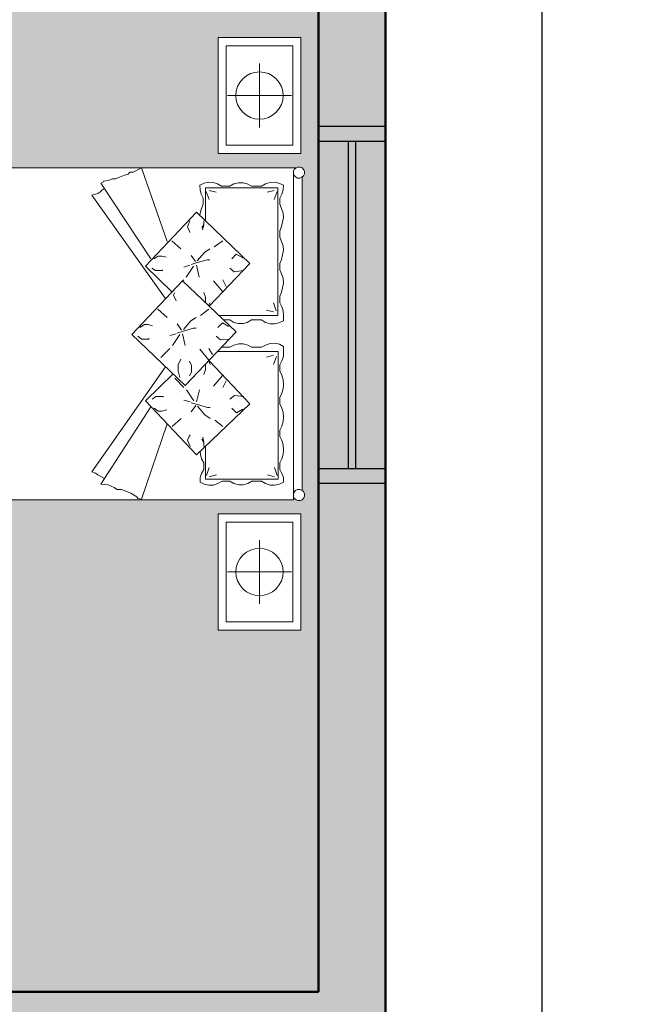
# Model space of a CAD drawing. Units: inches. Extents: x 528 to 2620, y -1066 to 798.
# Tile 33 of 41: x 1296 to 1381, y 524 to 656. Entities that reach past the tile are written whole.
import ezdxf

# ---------------------------------------------------------------- set-up
doc = ezdxf.new("R2010")
doc.units = ezdxf.units.IN
doc.header["$MEASUREMENT"] = 0
for name, color, linetype, lineweight in [('A-ANNO-DIMS', 2, 'Continuous', 18), ('A-FURN', 30, 'Continuous', 18), ('A-GLAZ', 3, 'Continuous', 25), ('A-WALL', 7, 'Continuous', 50), ('A-WALL-PATT', 8, 'Continuous', 13)]:
    doc.layers.add(name, color=color, linetype=linetype, lineweight=lineweight)
doc.styles.get("Standard").update_dxf_attribs({"font": 'arial.ttf'})
doc.dimstyles.get("Standard").update_dxf_attribs({"dimtxt": 6, "dimasz": 2, "dimexe": 0.18, "dimexo": 0.0625, "dimgap": 0.09, "dimtad": 0, "dimtih": 1, "dimtoh": 1, "dimdec": 1, "dimzin": 0, "dimdsep": 46, "dimlunit": 3, "dimtxsty": 'Standard', "dimblk": 'ARCHTICK', "dimcen": 0.09, "dimadec": 0, "dimazin": 0, "dimtfac": 1, "dimtdec": 1, "dimtofl": 0, "dimtmove": 0, "dimatfit": 3, "dimfxl": 1, "dimtolj": 1, "dimtzin": 0, "dimarcsym": 0})

# ---------------------------------------------------------------- blocks, each defined once
blk = doc.blocks.new('d-bed-3')
at = {"color": 0, "linetype": 'ByBlock'}
for p, q in [((0, 0), (0, -0.5)), ((0.7, 0), (0, 0)), ((0.7, -0.5), (0.7, 0)), ((0.7817, -0.0054), (0.7857, 0.0078)), ((0.7817, -0.0054), (0.7857, 0.0078)), ((0.7857, 0.0078), (0.7968, 0.0166)), ((0.7857, 0.0078), (0.7968, 0.0166)), ((0.7968, 0.0166), (0.8078, 0.0211)), ((0.7968, 0.0166), (0.8078, 0.0211)), ((0.8078, 0.0211), (0.8209, 0.0211)), ((0.8078, 0.0211), (0.8209, 0.0211)), ((0.8209, 0.0211), (0.8349, 0.0144)), ((0.8209, 0.0211), (0.8349, 0.0144)), ((0.8349, 0.0144), (0.8409, 0.0078)), ((0.8349, 0.0144), (0.8429, 0.0056)), ((0.8389, 0.0078), (2.7305, 0.0078)), ((0.8409, 0.0078), (2.7305, 0.0078)), ((0.8429, 0.0056), (0.848, -0.0077)), ((2.7234, -0.0077), (2.7284, 0.0056)), ((2.7284, 0.0056), (2.7365, 0.0144)), ((2.7305, 0.0078), (2.7365, 0.0144)), ((2.7365, 0.0144), (2.7505, 0.0211)), ((2.7365, 0.0144), (2.7505, 0.0211)), ((2.7505, 0.0211), (2.7636, 0.0211)), ((2.7505, 0.0211), (2.7636, 0.0211)), ((2.7636, 0.0211), (2.7746, 0.0166)), ((2.7636, 0.0211), (2.7746, 0.0166)), ((2.7746, 0.0166), (2.7857, 0.0078)), ((2.7746, 0.0166), (2.7857, 0.0078)), ((2.7857, 0.0078), (2.7897, -0.0054)), ((2.7857, 0.0078), (2.7897, -0.0054)), ((2.8714, -0.5), (2.8714, 0)), ((2.8714, 0), (3.5714, 0)), ((3.5714, 0), (3.5714, -0.5)), ((0.05, -0.05), (0.05, -0.45)), ((0.65, -0.05), (0.05, -0.05)), ((0.35, -0.0576), (0.35, -0.4424)), ((0.65, -0.45), (0.65, -0.05)), ((0.7817, -0.0187), (0.7817, -0.0054)), ((0.7817, -0.0187), (0.7817, -0.0054)), ((0.7857, -0.0297), (0.7817, -0.0187)), ((0.7857, -0.0297), (0.7817, -0.0187)), ((0.7857, -2.0939), (0.7857, -0.0297)), ((0.7948, -0.0408), (0.7857, -0.0297)), ((0.7857, -0.032), (0.7857, -2.0939)), ((0.8058, -0.0452), (0.7948, -0.0408)), ((0.8188, -0.0452), (0.8058, -0.0452)), ((0.8319, -0.0408), (0.8188, -0.0452)), ((2.7525, -0.0452), (0.8188, -0.0452)), ((0.8409, -0.032), (0.8319, -0.0408)), ((0.848, -0.0209), (0.8409, -0.032)), ((0.848, -0.0077), (0.848, -0.0209)), ((2.7234, -0.0209), (2.7234, -0.0077)), ((2.7305, -0.032), (2.7234, -0.0209)), ((2.7395, -0.0408), (2.7305, -0.032)), ((2.7525, -0.0452), (2.7395, -0.0408)), ((2.7656, -0.0452), (2.7525, -0.0452)), ((2.7766, -0.0408), (2.7656, -0.0452)), ((2.7766, -0.0408), (2.7656, -0.0452)), ((2.7656, -0.0452), (2.7857, -0.0452)), ((2.7857, -0.0452), (2.7656, -0.0452)), ((2.7857, -0.0297), (2.7766, -0.0408)), ((2.7857, -0.0297), (2.7766, -0.0408)), ((2.7897, -0.0187), (2.7857, -0.0297)), ((2.7897, -0.0187), (2.7857, -0.0297)), ((2.7857, -2.0939), (2.7857, -0.0452)), ((2.7897, -0.0054), (2.7897, -0.0187)), ((2.7897, -0.0054), (2.7897, -0.0187)), ((2.9214, -0.45), (2.9214, -0.05)), ((2.9214, -0.05), (3.5214, -0.05)), ((3.2214, -0.0576), (3.2214, -0.4424)), ((3.5214, -0.05), (3.5214, -0.45)), ((0.8781, -0.1325), (0.8911, -0.1059)), ((0.8911, -0.1059), (0.9182, -0.1082)), ((0.9182, -0.1082), (0.9443, -0.1148)), ((0.9443, -0.1148), (0.9684, -0.128)), ((1.0056, -0.128), (1.0317, -0.117)), ((1.0317, -0.117), (1.0588, -0.1082)), ((1.0588, -0.1082), (1.0849, -0.1059)), ((1.0849, -0.1059), (1.113, -0.1104)), ((1.113, -0.1104), (1.1401, -0.117)), ((1.1401, -0.117), (1.1662, -0.128)), ((1.2034, -0.128), (1.2295, -0.117)), ((1.2295, -0.117), (1.2566, -0.1082)), ((1.2566, -0.1082), (1.2827, -0.1059)), ((1.2827, -0.1059), (1.3108, -0.1104)), ((1.3108, -0.1104), (1.3379, -0.117)), ((1.3379, -0.117), (1.362, -0.128)), ((1.4012, -0.128), (1.4253, -0.117)), ((1.4253, -0.117), (1.4514, -0.1082)), ((1.4514, -0.1082), (1.4805, -0.1059)), ((1.4805, -0.1059), (1.5086, -0.1104)), ((1.5086, -0.1104), (1.5357, -0.117)), ((1.5357, -0.117), (1.5598, -0.128)), ((1.5989, -0.128), (1.623, -0.1148)), ((1.623, -0.1148), (1.6471, -0.1082)), ((1.6471, -0.1082), (1.6763, -0.1059)), ((1.6763, -0.1059), (1.7084, -0.1059)), ((1.7084, -0.1059), (1.7194, -0.1325)), ((1.8489, -0.1302), (1.863, -0.1059)), ((1.863, -0.1059), (1.8951, -0.1059)), ((1.8951, -0.1059), (1.9222, -0.1059)), ((1.9222, -0.1059), (1.9483, -0.1148)), ((1.9483, -0.1148), (1.9724, -0.128)), ((2.0096, -0.128), (2.0357, -0.1148)), ((2.0357, -0.1148), (2.0628, -0.1082)), ((2.0628, -0.1082), (2.0909, -0.1059)), ((2.0909, -0.1059), (2.117, -0.1082)), ((2.117, -0.1082), (2.1441, -0.1148)), ((2.1441, -0.1148), (2.1702, -0.128)), ((2.2074, -0.128), (2.2335, -0.1148)), ((2.2335, -0.1148), (2.2606, -0.1082)), ((2.2606, -0.1082), (2.2867, -0.1059)), ((2.2867, -0.1059), (2.3148, -0.1082)), ((2.3148, -0.1082), (2.3419, -0.1148)), ((2.3419, -0.1148), (2.366, -0.128)), ((2.4052, -0.128), (2.4293, -0.1148)), ((2.4293, -0.1148), (2.4554, -0.1082)), ((2.4554, -0.1082), (2.4845, -0.1059)), ((2.4845, -0.1059), (2.5126, -0.1082)), ((2.5126, -0.1082), (2.5397, -0.1148)), ((2.5397, -0.1148), (2.5638, -0.128)), ((2.6029, -0.128), (2.627, -0.1148)), ((2.627, -0.1148), (2.6511, -0.1059)), ((2.6511, -0.1059), (2.6803, -0.1059)), ((2.6803, -0.1059), (2.6913, -0.1302)), ((0.8721, -0.159), (0.8781, -0.1325)), ((0.8741, -0.1866), (0.8721, -0.159)), ((0.9072, -0.5753), (0.9072, -0.1391)), ((0.9072, -0.1391), (1.6763, -0.1391)), ((0.9223, -0.1612), (0.9333, -0.2042)), ((0.9293, -0.1435), (0.9775, -0.1612)), ((0.9684, -0.128), (1.0056, -0.128)), ((1.1662, -0.128), (1.2034, -0.128)), ((1.362, -0.128), (1.4012, -0.128)), ((1.5598, -0.128), (1.5989, -0.128)), ((1.6471, -0.1501), (1.5989, -0.1656)), ((1.6542, -0.1656), (1.6431, -0.2087)), ((1.6763, -0.1391), (1.6763, -0.4936)), ((1.7194, -0.1325), (1.7265, -0.159)), ((1.7265, -0.159), (1.7265, -0.1866)), ((1.8429, -0.159), (1.8489, -0.1302)), ((1.8449, -0.1866), (1.8429, -0.159)), ((2.6622, -0.1369), (1.8931, -0.1369)), ((1.8931, -0.1369), (1.8931, -0.5046)), ((1.9152, -0.1656), (1.9263, -0.2087)), ((1.9222, -0.1479), (1.9704, -0.1656)), ((1.9724, -0.128), (2.0096, -0.128)), ((2.1702, -0.128), (2.2074, -0.128)), ((2.366, -0.128), (2.4052, -0.128)), ((2.5638, -0.128), (2.6029, -0.128)), ((2.6401, -0.1435), (2.5919, -0.159)), ((2.6471, -0.159), (2.6361, -0.202)), ((2.6622, -0.5753), (2.6622, -0.1369)), ((2.6913, -0.1302), (2.6973, -0.159)), ((2.6973, -0.159), (2.6973, -0.1866)), ((0.8831, -0.2131), (0.8741, -0.1866)), ((0.8962, -0.2374), (0.8831, -0.2131)), ((1.7174, -0.2131), (1.7024, -0.2374)), ((1.7265, -0.1866), (1.7174, -0.2131)), ((1.854, -0.2131), (1.8449, -0.1866)), ((1.867, -0.2374), (1.854, -0.2131)), ((2.6883, -0.2131), (2.6732, -0.2374)), ((2.6973, -0.1866), (2.6883, -0.2131)), ((0.1576, -0.25), (0.5424, -0.25)), ((0.8962, -0.2992), (0.8962, -0.2374)), ((1.7024, -0.2374), (1.7024, -0.2992)), ((1.867, -0.297), (1.867, -0.2374)), ((2.6732, -0.2374), (2.6732, -0.297)), ((3.4138, -0.25), (3.029, -0.25)), ((0.8761, -0.3489), (0.8831, -0.3235)), ((0.8761, -0.3776), (0.8761, -0.3489)), ((0.8831, -0.3235), (0.8962, -0.2992)), ((1.0538, -0.6294), (1.362, -0.3081)), ((1.3289, -0.3511), (1.3068, -0.3909)), ((1.362, -0.3081), (1.619, -0.5532)), ((1.4052, -0.3467), (1.4122, -0.4019)), ((1.7024, -0.2992), (1.7174, -0.3235)), ((1.7174, -0.3235), (1.7244, -0.3489)), ((1.7244, -0.3489), (1.7244, -0.3776)), ((1.8469, -0.3489), (1.854, -0.3213)), ((1.8469, -0.3754), (1.8469, -0.3489)), ((1.854, -0.3213), (1.867, -0.297)), ((2.2074, -0.3081), (1.9483, -0.5532)), ((2.1632, -0.3445), (2.1572, -0.3997)), ((2.5146, -0.6294), (2.2074, -0.3081)), ((2.2405, -0.3511), (2.2626, -0.3887)), ((2.6732, -0.297), (2.6883, -0.3213)), ((2.6883, -0.3213), (2.6953, -0.3489)), ((2.6953, -0.3489), (2.6953, -0.3754)), ((0.8831, -0.4041), (0.8761, -0.3776)), ((0.8962, -0.4284), (0.8831, -0.4041)), ((1.3068, -0.3909), (1.3349, -0.4174)), ((1.4122, -0.4019), (1.3901, -0.4284)), ((1.4674, -0.7134), (1.7746, -0.3909)), ((1.7174, -0.4041), (1.7024, -0.4284)), ((1.7244, -0.3776), (1.7174, -0.4041)), ((1.7746, -0.3909), (2.0979, -0.6979)), ((1.854, -0.4041), (1.8469, -0.3754)), ((1.867, -0.4284), (1.854, -0.4041)), ((2.1572, -0.3997), (2.1793, -0.4284)), ((2.2626, -0.3887), (2.2335, -0.4174)), ((2.6883, -0.4041), (2.6732, -0.4284)), ((2.6953, -0.3754), (2.6883, -0.4041)), ((0.05, -0.45), (0.65, -0.45)), ((0.8962, -0.4781), (0.8962, -0.4284)), ((1.2255, -0.4715), (1.2626, -0.5223)), ((1.5006, -0.4505), (1.4604, -0.4715)), ((1.5327, -0.4715), (1.4674, -0.5267)), ((1.7024, -0.4284), (1.7024, -0.4649)), ((1.7415, -0.4351), (1.7194, -0.4737)), ((1.7194, -0.4737), (1.7485, -0.5002)), ((1.8188, -0.4306), (1.8228, -0.4848)), ((1.867, -0.4781), (1.867, -0.4284)), ((2.0357, -0.4715), (2.102, -0.5267)), ((2.0688, -0.4505), (2.109, -0.4715)), ((2.3439, -0.4715), (2.3068, -0.5201)), ((2.6732, -0.4284), (2.6732, -0.4759)), ((3.5214, -0.45), (2.9214, -0.45)), ((0, -0.5), (0.7, -0.5)), ((0.8721, -0.5576), (0.8741, -0.5289)), ((0.8741, -0.5289), (0.8831, -0.5024)), ((0.8831, -0.5024), (0.8962, -0.4781)), ((0.9223, -0.5532), (0.9333, -0.5113)), ((1.8228, -0.4848), (1.8008, -0.5113)), ((1.9112, -0.5333), (1.874, -0.5554)), ((2.6471, -0.5532), (2.6361, -0.5091)), ((2.6732, -0.4759), (2.6883, -0.5002)), ((2.6883, -0.5002), (2.6973, -0.5267)), ((2.6973, -0.5267), (2.6973, -0.5554)), ((3.5714, -0.5), (2.8714, -0.5)), ((0.8781, -0.5841), (0.8721, -0.5576)), ((0.8911, -0.6096), (0.8781, -0.5841)), ((1.109, -0.5753), (0.9072, -0.5753)), ((0.9293, -0.5709), (0.9775, -0.5532)), ((0.9684, -0.5886), (0.9443, -0.6007)), ((1.0056, -0.5886), (0.9684, -0.5886)), ((1.0317, -0.5996), (1.0056, -0.5886)), ((1.105, -0.5864), (1.1271, -0.5864)), ((1.1271, -0.5864), (1.1482, -0.5974)), ((1.1482, -0.5974), (1.1311, -0.5864)), ((1.1311, -0.5864), (1.1592, -0.593)), ((1.2957, -0.5819), (1.2737, -0.5488)), ((1.3459, -0.625), (1.2957, -0.5819)), ((1.3399, -0.5643), (1.3399, -0.5488)), ((1.357, -0.625), (1.3399, -0.5643)), ((1.5658, -0.5753), (1.5377, -0.5864)), ((1.5969, -0.5753), (1.5658, -0.5753)), ((1.5989, -0.5488), (1.614, -0.5554)), ((1.6381, -0.5554), (1.6763, -0.6051)), ((1.9443, -0.5554), (1.8781, -0.6096)), ((1.9704, -0.5466), (1.9503, -0.5554)), ((1.9684, -0.5753), (2.0036, -0.5753)), ((2.0036, -0.5753), (2.0317, -0.5864)), ((2.2124, -0.6228), (2.2295, -0.5643)), ((2.2224, -0.6228), (2.2736, -0.5797)), ((2.2295, -0.5643), (2.2295, -0.5466)), ((2.2736, -0.5797), (2.2957, -0.5466)), ((2.4383, -0.5864), (2.4092, -0.5908)), ((2.4423, -0.5864), (2.4202, -0.5974)), ((2.4202, -0.5974), (2.4383, -0.5864)), ((2.4644, -0.5864), (2.4423, -0.5864)), ((2.4604, -0.5753), (2.6622, -0.5753)), ((2.5638, -0.5864), (2.5397, -0.5996)), ((2.6029, -0.5864), (2.5638, -0.5864)), ((2.6401, -0.5687), (2.5919, -0.5532)), ((2.627, -0.5996), (2.6029, -0.5864)), ((2.6913, -0.5841), (2.6803, -0.6073)), ((2.6973, -0.5554), (2.6913, -0.5841)), ((0.9182, -0.6073), (0.8911, -0.6096)), ((0.9443, -0.6007), (0.9182, -0.6073)), ((1.0588, -0.6073), (1.0317, -0.5996)), ((1.3791, -0.9365), (1.0538, -0.6294)), ((1.0759, -0.6096), (1.0588, -0.6073)), ((1.3138, -0.6626), (1.351, -0.6361)), ((1.368, -0.6626), (1.357, -0.625)), ((1.3731, -0.6294), (1.4453, -0.614)), ((1.3791, -0.6471), (1.4453, -0.6913)), ((1.7084, -0.6648), (1.6873, -0.6316)), ((1.7526, -0.6493), (1.7526, -0.6316)), ((1.7706, -0.7089), (1.7526, -0.6493)), ((2.0387, -0.6427), (2.0427, -0.6405)), ((2.1963, -0.6294), (2.124, -0.6118)), ((2.1903, -0.6449), (2.124, -0.6891)), ((2.1903, -0.9365), (2.5146, -0.6294)), ((2.2013, -0.6626), (2.2124, -0.6228)), ((2.2556, -0.6626), (2.2184, -0.6338)), ((2.5126, -0.6051), (2.4955, -0.6073)), ((2.5397, -0.5996), (2.5126, -0.6051)), ((2.6511, -0.6073), (2.627, -0.5996)), ((2.6803, -0.6073), (2.6511, -0.6073)), ((1.105, -0.6692), (1.1421, -0.6846)), ((1.1421, -0.6846), (1.1642, -0.6736)), ((1.1642, -0.6736), (1.1753, -0.6692)), ((1.3731, -0.6692), (1.3841, -0.7067)), ((1.4674, -0.7134), (1.4604, -0.7067)), ((1.7596, -0.7089), (1.7084, -0.6648)), ((1.7817, -0.7454), (1.7706, -0.7089)), ((1.7857, -0.7134), (1.856, -0.6979)), ((2.0979, -0.6979), (1.7897, -1.0193)), ((1.9765, -0.6604), (1.9503, -0.6714)), ((2.0166, -0.6604), (1.9765, -0.6604)), ((2.0387, -0.6714), (2.0166, -0.6604)), ((2.0538, -0.7609), (2.109, -0.7067)), ((2.1963, -0.667), (2.1853, -0.7067)), ((2.4052, -0.6736), (2.3941, -0.667)), ((2.4272, -0.6846), (2.4052, -0.6736)), ((2.4644, -0.667), (2.4272, -0.6846)), ((1.2255, -0.7785), (1.2737, -0.7244)), ((1.7897, -1.0193), (1.4674, -0.7134)), ((1.5548, -0.7675), (1.5397, -0.7631)), ((1.5548, -0.7675), (1.5769, -0.7564)), ((1.5769, -0.7564), (1.5879, -0.752)), ((1.7265, -0.7454), (1.7636, -0.72)), ((1.7857, -0.752), (1.7967, -0.7896)), ((1.7897, -0.731), (1.856, -0.7741)), ((1.9724, -0.741), (1.9393, -0.7244)), ((2.0096, -0.741), (1.9724, -0.741)), ((2.0497, -0.731), (2.0096, -0.741)), ((2.1903, -0.9365), (2.0277, -0.7697)), ((2.3439, -0.7763), (2.2957, -0.7222)), ((0.7857, -0.9607), (1.2295, -0.8072)), ((0.9504, -1.2611), (1.5708, -0.8183)), ((1.3178, -0.8382), (1.3239, -0.8117)), ((1.3791, -0.9365), (1.5357, -0.7763)), ((1.6381, -0.8625), (1.6873, -0.8072)), ((1.9283, -0.8448), (1.874, -0.7896)), ((2.618, -1.2611), (1.9855, -0.8161)), ((2.2515, -0.8382), (2.2445, -0.8094)), ((2.7827, -0.9607), (2.3278, -0.8072)), ((1.3178, -0.8602), (1.3178, -0.8382)), ((1.3349, -0.8879), (1.3178, -0.8602)), ((1.3901, -0.8989), (1.4052, -0.8768)), ((1.4052, -0.8337), (1.4012, -0.8337)), ((1.4052, -0.8768), (1.4052, -0.8337)), ((2.1632, -0.8757), (2.1632, -0.8315)), ((2.1632, -0.8315), (2.1682, -0.8315)), ((2.1793, -0.8967), (2.1632, -0.8757)), ((2.2335, -0.8856), (2.2515, -0.8602)), ((2.2515, -0.8602), (2.2515, -0.8382)), ((0.8781, -1.2059), (1.3349, -0.9055)), ((1.7305, -0.921), (1.7375, -0.8945)), ((1.7305, -0.9431), (1.7305, -0.921)), ((1.7485, -0.9718), (1.7305, -0.9431)), ((1.8188, -0.9166), (1.8118, -0.9166)), ((1.8188, -0.9607), (1.8188, -0.9166)), ((2.6913, -1.2059), (2.2254, -0.9055)), ((0.8128, -1.0115), (0.7857, -0.9607)), ((1.8008, -0.9828), (1.8188, -0.9607)), ((2.7676, -0.9895), (2.7455, -1.0259)), ((2.7786, -0.9828), (2.7676, -0.9895)), ((2.7827, -0.9607), (2.7786, -0.9828)), ((0.8128, -1.0325), (0.8128, -1.0115)), ((0.8239, -1.0414), (0.8128, -1.0325)), ((0.8299, -1.0635), (0.8239, -1.0414)), ((0.8349, -1.0745), (0.8299, -1.0635)), ((2.7455, -1.0259), (2.7234, -1.0811)), ((0.845, -1.1032), (0.8349, -1.0745)), ((0.852, -1.1187), (0.845, -1.1032)), ((0.852, -1.1363), (0.852, -1.1187)), ((2.7124, -1.1253), (2.6953, -1.1617)), ((2.7174, -1.1187), (2.7124, -1.1253)), ((2.7234, -1.1076), (2.7174, -1.1187)), ((2.7234, -1.0811), (2.7234, -1.1076)), ((0.863, -1.1617), (0.852, -1.1363)), ((0.867, -1.1905), (0.863, -1.1617)), ((0.9223, -1.2015), (0.9112, -1.1838)), ((2.6582, -1.1838), (2.6471, -1.2015)), ((2.6953, -1.1617), (2.6913, -1.2059)), ((0.8741, -1.1949), (0.867, -1.1905)), ((0.8781, -1.2059), (0.8741, -1.1949)), ((0.9293, -1.2059), (0.9223, -1.2015)), ((0.9403, -1.2236), (0.9293, -1.2059)), ((0.9443, -1.2391), (0.9403, -1.2236)), ((0.9504, -1.2611), (0.9443, -1.2391)), ((2.625, -1.2391), (2.618, -1.2611)), ((2.6361, -1.2236), (2.625, -1.2391)), ((2.6471, -1.2015), (2.6361, -1.2236)), ((2.7234, -2.0497), (2.6913, -1.947)), ((0.8741, -2.0673), (0.9464, -1.9691)), ((0.8851, -2.1005), (0.9795, -2.0342)), ((2.7305, -2.0939), (2.6421, -2.0342)), ((0.7797, -2.148), (0.7857, -2.1347)), ((0.7797, -2.148), (0.7857, -2.1347)), ((0.7888, -2.1317), (0.7857, -2.0939)), ((0.7857, -2.0939), (0.7887, -2.1303)), ((0.7857, -2.1347), (0.7948, -2.1259)), ((0.7857, -2.1347), (0.7888, -2.1317)), ((0.7948, -2.1259), (0.8078, -2.1215)), ((0.8078, -2.1215), (0.8188, -2.1215)), ((0.8188, -2.1215), (0.8319, -2.1281)), ((0.8319, -2.1281), (0.8409, -2.1369)), ((2.7365, -2.1281), (2.7284, -2.1369)), ((2.7505, -2.1215), (2.7365, -2.1281)), ((2.7616, -2.1215), (2.7505, -2.1215)), ((2.7746, -2.1259), (2.7616, -2.1215)), ((2.7827, -2.1347), (2.7746, -2.1259)), ((2.7857, -2.0939), (2.7783, -2.1299)), ((2.7783, -2.1299), (2.7827, -2.1347)), ((2.7786, -2.1281), (2.7857, -2.0939)), ((2.7827, -2.1347), (2.7897, -2.148)), ((2.7897, -2.148), (2.7827, -2.1347)), ((0.7797, -2.159), (0.7797, -2.148)), ((0.7797, -2.148), (0.7797, -2.159)), ((0.7837, -2.1723), (0.7797, -2.159)), ((0.7837, -2.1723), (0.7797, -2.159)), ((0.7927, -2.1811), (0.7837, -2.1723)), ((0.7927, -2.1811), (0.7837, -2.1723)), ((0.8058, -2.1877), (0.7927, -2.1811)), ((0.8058, -2.1877), (0.7927, -2.1811)), ((0.8168, -2.1877), (0.8058, -2.1877)), ((0.8168, -2.1877), (0.8058, -2.1877)), ((0.8299, -2.1833), (0.8168, -2.1877)), ((0.8299, -2.1833), (0.8168, -2.1877)), ((0.8389, -2.1745), (0.8299, -2.1833)), ((0.8367, -2.1767), (0.8299, -2.1833)), ((2.7327, -2.1767), (0.8367, -2.1767)), ((0.845, -2.1612), (0.8389, -2.1745)), ((0.8389, -2.1767), (2.7305, -2.1767)), ((0.8409, -2.1369), (0.845, -2.1502)), ((2.7264, -2.1436), (0.845, -2.1436)), ((0.845, -2.1502), (0.845, -2.1612)), ((2.7284, -2.1369), (2.7234, -2.1502)), ((2.7234, -2.1502), (2.7234, -2.1612)), ((2.7234, -2.1612), (2.7305, -2.1745)), ((2.7305, -2.1745), (2.7395, -2.1833)), ((2.7395, -2.1833), (2.7327, -2.1767)), ((2.7525, -2.1877), (2.7395, -2.1833)), ((2.7395, -2.1833), (2.7525, -2.1877)), ((2.7636, -2.1877), (2.7525, -2.1877)), ((2.7525, -2.1877), (2.7636, -2.1877)), ((2.7766, -2.1811), (2.7636, -2.1877)), ((2.7636, -2.1877), (2.7766, -2.1811)), ((2.7857, -2.1723), (2.7766, -2.1811)), ((2.7766, -2.1811), (2.7857, -2.1723)), ((2.7897, -2.159), (2.7857, -2.1723)), ((2.7857, -2.1723), (2.7897, -2.159)), ((2.7897, -2.148), (2.7897, -2.159)), ((2.7897, -2.159), (2.7897, -2.148))]:
    blk.add_line(p, q, dxfattribs=at)
blk.add_ellipse((0.35, -0.25), major_axis=(-0.1007, 0.1007), ratio=1, dxfattribs=at)
at = {"color": 0, "linetype": 'ByBlock', "extrusion": (0, 0, -1)}
blk.add_ellipse((3.2214, -0.25), major_axis=(0.1007, 0.1007), ratio=1, dxfattribs=at)
blk = doc.blocks.new('_ArchTick')
at = {"color": 0, "linetype": 'ByBlock', "const_width": 0.15}
blk.add_lwpolyline([(-0.5, -0.5), (0.5, 0.5)], dxfattribs=at)
blk = doc.blocks.new('*D17')
at = {"layer": 'A-ANNO-DIMS', "color": 0, "lineweight": -2, "transparency": 16777216}
for p, q in [((1345.06, 718.92), (1366.18, 718.92)), ((1366, 718.92), (1366, 497.08)), ((1366, 268.92), (1366, 490.77)), ((1345.06, 268.92), (1366.18, 268.92))]:
    blk.add_line(p, q, dxfattribs=at)
at = {"layer": 'Defpoints', "color": 0, "transparency": 16777216}
for p in [(1345, 718.92), (1345, 268.92), (1366, 268.92)]:
    blk.add_point(p, dxfattribs=at)
at = {"layer": 'A-ANNO-DIMS', "color": 0, "lineweight": -2, "transparency": 16777216, "xscale": 2, "yscale": 2, "zscale": 2}
for p, rotation in [((1366, 718.92), 90), ((1366, 268.92), 270)]:
    blk.add_blockref('_ArchTick', p, dxfattribs=dict(at, rotation=rotation))
at = {"layer": 'A-ANNO-DIMS', "color": 0, "transparency": 16777216, "insert": (1366, 493.92), "char_height": 6, "attachment_point": 5}
blk.add_mtext('\\A1;37\'-6.0"', dxfattribs=at)
blk = doc.blocks.new('WIN-1200')
for p, q in [((677.56, 718.92), (725.56, 718.92)), ((677.56, 709.92), (677.56, 718.92)), ((679.56, 709.92), (679.56, 718.92)), ((723.56, 718.92), (723.56, 709.92)), ((725.56, 718.92), (725.56, 709.92)), ((679.56, 714.92), (723.56, 714.92)), ((679.56, 713.92), (723.56, 713.92)), ((725.56, 709.92), (677.56, 709.92))]:
    blk.add_line(p, q)

msp = doc.modelspace()

# ---------------------------------------------------------------- hatches: boundary and pattern name
at = {"layer": 'A-WALL-PATT', "transparency": 33554521}
h = msp.add_hatch(color=256, dxfattribs=at)
h.dxf.hatch_style = 1
h.paths.add_polyline_path([(1066, 709.92), (1114.5, 709.92), (1114.5, 718.92), (1057, 718.92), (1057, 667.92), (1066, 667.92)])
h.paths.add_polyline_path([(1227.5, 718.92), (1162.5, 718.92), (1162.5, 709.92), (1211, 709.92), (1211, 577.92), (1205.42, 577.92), (1205.5, 573.42), (1211, 573.42), (1211, 567.42), (1215.5, 567.42), (1215.5, 669.42), (1268, 669.42), (1268, 675.92), (1263.5, 675.92), (1263.5, 673.92), (1215.5, 673.92), (1215.5, 709.92), (1227.5, 709.92)])
h.paths.add_polyline_path([(1345, 718.92), (1316, 718.92), (1316, 709.92), (1336, 709.92), (1336, 641.67), (1345, 641.67)])
h.paths.add_polyline_path([(1066, 619.92), (1057, 619.92), (1057, 561.42), (1066, 561.42), (1066, 573.42), (1161, 573.42), (1161, 569.42), (1165.5, 569.42), (1165.5, 577.92), (1066, 577.92)])
h.paths.add_polyline_path([(1216, 391.42), (1216, 400.42), (1207, 400.42), (1201, 400.42), (1201, 397.42), (1201, 391.42), (1207, 391.42), (1207, 268.92), (1252, 268.92), (1252, 277.92), (1216, 277.92), (1216, 359.77)])
h.paths.add_polyline_path([(1345, 395.92), (1336, 395.92), (1288, 395.92), (1288, 391.42), (1336, 391.42), (1336, 277.92), (1300, 277.92), (1300, 268.92), (1345, 268.92)])
h.paths.add_polyline_path([(1345, 593.67), (1336, 593.67), (1336, 525.42), (1215.5, 525.42), (1215.5, 527.17), (1211, 527.17), (1211, 520.92), (1336, 520.92), (1336, 443.92), (1345, 443.92)])
h.paths.add_polyline_path([(1066, 520.92), (1165.5, 520.92), (1165.5, 545.42), (1161, 545.42), (1161, 525.42), (1066, 525.42), (1066, 537.42), (1057, 537.42), (1057, 484.67), (1066, 484.67)])
h.paths.add_polyline_path([(1066, 436.67), (1057, 436.67), (1057, 391.42), (1085.5, 391.42), (1085.5, 400.42), (1066, 400.42)])
h.paths.add_polyline_path([(1153, 397.42), (1153, 400.42), (1133.5, 400.42), (1133.5, 391.42), (1153, 391.42)])
at = {"layer": 'A-WALL-PATT', "transparency": 33554681}
h = msp.add_hatch(color=256, dxfattribs=at)
h.dxf.hatch_style = 1
h.paths.add_polyline_path([(1066, 665.92), (1062, 665.92), (1062, 621.92), (1066, 621.92)])
h.paths.add_polyline_path([(1061, 665.92), (1057, 665.92), (1057, 621.92), (1061, 621.92)])
h.paths.add_polyline_path([(1160.5, 713.92), (1116.5, 713.92), (1116.5, 709.92), (1160.5, 709.92)])
h.paths.add_polyline_path([(1160.5, 718.92), (1116.5, 718.92), (1116.5, 714.92), (1160.5, 714.92)])
h.paths.add_polyline_path([(1251.5, 713.92), (1227.5, 713.92), (1227.5, 709.92), (1251.5, 709.92)])
h.paths.add_polyline_path([(1251.5, 718.92), (1227.5, 718.92), (1227.5, 714.92), (1251.5, 714.92)])
h.paths.add_polyline_path([(1314, 713.92), (1270, 713.92), (1270, 709.92), (1314, 709.92)])
h.paths.add_polyline_path([(1314, 718.92), (1270, 718.92), (1270, 714.92), (1314, 714.92)])
h.paths.add_polyline_path([(1345, 639.67), (1341, 639.67), (1341, 595.67), (1345, 595.67)])
h.paths.add_polyline_path([(1340, 639.67), (1336, 639.67), (1336, 595.67), (1340, 595.67)])
h.paths.add_polyline_path([(1345, 441.92), (1341, 441.92), (1341, 397.92), (1345, 397.92)])
h.paths.add_polyline_path([(1340, 441.92), (1336, 441.92), (1336, 397.92), (1340, 397.92)])
h.paths.add_polyline_path([(1298, 272.92), (1254, 272.92), (1254, 268.92), (1298, 268.92)])
h.paths.add_polyline_path([(1298, 277.92), (1254, 277.92), (1254, 273.92), (1298, 273.92)])
h.paths.add_polyline_path([(1131.5, 395.42), (1087.5, 395.42), (1087.5, 391.42), (1131.5, 391.42)])
h.paths.add_polyline_path([(1131.5, 400.42), (1087.5, 400.42), (1087.5, 396.42), (1131.5, 396.42)])
h.paths.add_polyline_path([(1066, 482.67), (1062, 482.67), (1062, 438.67), (1066, 438.67)])
h.paths.add_polyline_path([(1061, 482.67), (1057, 482.67), (1057, 438.67), (1061, 438.67)])
h.paths.add_polyline_path([(1066, 561.42), (1062, 561.42), (1062, 537.42), (1066, 537.42)])
h.paths.add_polyline_path([(1061, 561.42), (1057, 561.42), (1057, 537.42), (1061, 537.42)])
at = {"layer": 'A-WALL-PATT', "transparency": 33554536}
h = msp.add_hatch(color=256, dxfattribs=at)
h.dxf.hatch_style = 1
h.paths.add_polyline_path([(1336, 709.92), (1268, 709.92), (1268, 699.92), (1266.75, 699.92), (1266.75, 675.92), (1268, 675.92), (1268, 669.42), (1215.5, 669.42), (1215.5, 567.17), (1217, 567.17), (1257, 567.17), (1257, 565.42), (1256.96, 565.42, -0.401453), (1217, 527.17), (1215.5, 527.17), (1215.5, 525.42), (1336, 525.42)], flags=17)
h.paths.add_polyline_path([(1285.03, 635.93), (1285.23, 636.13), (1285.67, 636.26), (1286.21, 636.02), (1286.98, 636.08), (1332.98, 636.08), (1333.36, 636.22), (1333.82, 636.08), (1334.11, 635.71), (1334.11, 635.3), (1333.91, 634.86), (1333.82, 634.83), (1333.82, 592.74), (1333.97, 592.6), (1334.11, 592.29), (1334.11, 591.88), (1333.82, 591.51), (1333.36, 591.37), (1332.98, 591.51), (1332.64, 591.79), (1332.64, 591.51), (1286.98, 591.51), (1286.17, 591.67), (1286.07, 591.57), (1285.68, 591.37), (1285.23, 591.51), (1285.03, 591.71), (1284.83, 592.1), (1284.98, 592.54), (1285.13, 592.69), (1285.13, 634.95), (1284.98, 635.1), (1284.83, 635.54)], flags=16)
h.paths.add_polyline_path([(1285.03, 635.93), (1285.23, 636.13), (1285.67, 636.26), (1286.21, 636.02), (1286.98, 636.08), (1332.98, 636.08), (1333.36, 636.22), (1333.82, 636.08), (1334.11, 635.71), (1334.11, 635.3), (1333.97, 634.99), (1333.82, 634.85), (1333.82, 592.74), (1333.97, 592.6), (1334.11, 592.29), (1334.11, 591.88), (1333.82, 591.51), (1333.36, 591.37), (1332.98, 591.51), (1332.64, 591.79), (1332.64, 592.25), (1332.64, 635.35), (1332.64, 635.8), (1332.98, 636.08), (1312.23, 636.08), (1311.1, 635.48), (1310.63, 635.48), (1310.43, 635.23), (1309.94, 635.1), (1309.7, 634.99), (1309.06, 634.76), (1308.71, 634.61), (1308.32, 634.61), (1307.75, 634.36), (1307.11, 634.27), (1307.01, 634.11), (1306.77, 634.02), (1307.25, 633.28), (1306.87, 633.04), (1306.77, 632.88), (1306.37, 632.64), (1306.03, 632.55), (1305.54, 632.41), (1315.47, 618.49), (1316.32, 619.39), (1312.77, 622.86), (1319.62, 630.11), (1320.07, 629.68), (1320.11, 630), (1320.28, 630.6), (1320.53, 631.18), (1320.53, 632.01), (1320.26, 632.55), (1320.11, 633.13), (1320.06, 633.73), (1320.63, 634.02), (1321.22, 634.16), (1321.86, 634.11), (1322.45, 633.91), (1322.99, 633.62), (1324.1, 633.62), (1324.64, 633.91), (1325.23, 634.07), (1325.87, 634.07), (1326.43, 633.91), (1326.98, 633.62), (1328.35, 633.62), (1328.9, 633.91), (1329.49, 634.11), (1330.1, 634.16), (1330.69, 634.02), (1331.28, 633.73), (1331.23, 633.13), (1331.09, 632.55), (1330.79, 632.01), (1330.79, 631.18), (1331.04, 630.6), (1331.23, 630), (1331.28, 629.41), (1331.19, 628.79), (1331.04, 628.18), (1330.79, 627.6), (1330.79, 626.77), (1331.04, 626.19), (1331.23, 625.59), (1331.28, 625.01), (1331.19, 624.38), (1331.04, 623.78), (1330.79, 623.24), (1330.79, 622.37), (1331.04, 621.83), (1331.23, 621.25), (1331.28, 620.6), (1331.19, 619.97), (1331.04, 619.37), (1330.79, 618.83), (1330.79, 617.96), (1331.09, 617.42), (1331.23, 616.88), (1331.28, 616.23), (1331.28, 615.52), (1330.69, 615.27), (1330.1, 615.12), (1329.49, 615.12), (1328.9, 615.32), (1328.35, 615.65), (1326.98, 615.65), (1326.43, 615.32), (1325.87, 615.16), (1325.23, 615.16), (1324.64, 615.32), (1324.1, 615.65), (1323.24, 615.65), (1324.93, 614.04), (1322.98, 611.98), (1324.1, 611.98), (1324.64, 612.27), (1325.28, 612.43), (1325.87, 612.43), (1326.48, 612.27), (1327.03, 611.98), (1328.35, 611.98), (1328.9, 612.27), (1329.49, 612.48), (1330.1, 612.52), (1330.74, 612.39), (1331.28, 612.07), (1331.28, 611.36), (1331.28, 610.75), (1331.09, 610.17), (1330.79, 609.63), (1330.79, 608.81), (1331.09, 608.22), (1331.23, 607.62), (1331.28, 606.99), (1331.23, 606.41), (1331.09, 605.81), (1330.79, 605.22), (1330.79, 604.4), (1331.09, 603.81), (1331.23, 603.21), (1331.28, 602.63), (1331.23, 602), (1331.09, 601.4), (1330.79, 600.86), (1330.79, 599.99), (1331.09, 599.45), (1331.23, 598.87), (1331.28, 598.22), (1331.23, 597.59), (1331.09, 596.99), (1330.79, 596.45), (1330.79, 595.58), (1331.09, 595.04), (1331.28, 594.51), (1331.28, 593.86), (1330.74, 593.61), (1330.1, 593.48), (1329.49, 593.48), (1328.9, 593.68), (1328.35, 594.01), (1327.03, 594.01), (1326.48, 593.68), (1325.87, 593.52), (1325.28, 593.52), (1324.64, 593.68), (1324.1, 594.01), (1323.04, 594.01), (1322.5, 593.68), (1321.91, 593.48), (1321.27, 593.48), (1320.63, 593.61), (1320.11, 593.86), (1320.11, 594.51), (1320.28, 595.04), (1320.58, 595.58), (1320.58, 596.45), (1320.28, 596.99), (1320.16, 597.59), (1320.1, 598.01), (1319.62, 597.55), (1315.66, 601.73), (1312.23, 591.57), (1311.74, 591.66), (1311.59, 591.91), (1310.78, 592.4), (1309.55, 592.89), (1308.96, 592.89), (1308.71, 593.03), (1308.56, 593.14), (1307.75, 593.52), (1306.77, 593.61), (1307.25, 594.36), (1306.87, 594.6), (1306.37, 594.84), (1306.03, 595.09), (1305.54, 595.24), (1315.46, 609.35), (1310.93, 613.71), (1315.47, 618.49), (1305.54, 632.41), (1306.03, 632.55), (1306.37, 632.64), (1306.77, 632.88), (1306.87, 633.04), (1307.25, 633.28), (1306.77, 634.02), (1307.01, 634.11), (1307.11, 634.27), (1307.75, 634.36), (1308.32, 634.61), (1308.71, 634.61), (1309.06, 634.76), (1309.7, 634.99), (1309.94, 635.1), (1310.43, 635.23), (1310.63, 635.48), (1311.1, 635.48), (1312.23, 636.08), (1286.98, 636.08), (1286.22, 636.02), (1286.41, 635.44), (1286.21, 635.05), (1286.02, 634.85), (1285.87, 634.81), (1285.87, 592.84), (1286.15, 592.73), (1286.41, 592.19), (1286.23, 591.66), (1286.17, 591.67), (1286.07, 591.57), (1285.68, 591.37), (1285.23, 591.51), (1285.03, 591.71), (1284.83, 592.1), (1284.98, 592.54), (1285.13, 592.69), (1285.13, 634.95), (1284.98, 635.1), (1284.83, 635.54)], flags=0)
h.paths.add_polyline_path([(1322.5, 653.6), (1333.65, 653.6), (1333.65, 637.99), (1322.5, 637.99)], flags=16)
h.paths.add_polyline_path([(1323.62, 652.48), (1332.53, 652.48), (1332.53, 639.11), (1323.62, 639.11)], flags=0)
edge = h.paths.add_edge_path(flags=0)
edge.add_ellipse((1328.07, 645.79), major_axis=(2.24, 2.24), ratio=1, start_angle=405, end_angle=495, ccw=False)
edge.add_ellipse((1328.07, 645.79), major_axis=(2.24, 2.24), ratio=1, start_angle=675, end_angle=765, ccw=False)
edge.add_ellipse((1328.07, 645.79), major_axis=(2.24, 2.24), ratio=1, start_angle=585, end_angle=675, ccw=False)
edge.add_ellipse((1328.07, 645.79), major_axis=(2.24, 2.24), ratio=1, start_angle=495, end_angle=585, ccw=False)
h.paths.add_polyline_path([(1320.58, 628.39), (1320.33, 628.01), (1320.61, 628.55)], flags=0)
h.paths.add_polyline_path([(1317.89, 604.89), (1318.78, 604.64), (1319.76, 604.28), (1318.88, 604.53)], flags=0)
h.paths.add_polyline_path([(1320.33, 599.65), (1320.58, 599.25), (1320.58, 599.16)], flags=0)
h.paths.add_polyline_path([(1322.5, 589.6), (1333.65, 589.6), (1333.65, 573.99), (1322.5, 573.99)], flags=16)
h.paths.add_polyline_path([(1323.62, 588.48), (1332.53, 588.48), (1332.53, 575.11), (1323.62, 575.11)], flags=0)
edge = h.paths.add_edge_path(flags=0)
edge.add_ellipse((1328.07, 581.8), major_axis=(-2.24, 2.24), ratio=1, start_angle=-45, end_angle=45, ccw=False)
edge.add_ellipse((1328.07, 581.8), major_axis=(-2.24, 2.24), ratio=1, start_angle=-135, end_angle=-45, ccw=False)
edge.add_ellipse((1328.07, 581.8), major_axis=(-2.24, 2.24), ratio=1, start_angle=135, end_angle=-135, ccw=False)
edge.add_ellipse((1328.07, 581.8), major_axis=(-2.24, 2.24), ratio=1, start_angle=45, end_angle=135, ccw=False)
h.paths.add_polyline_path([(1264.75, 699.92), (1263.5, 699.92), (1263.5, 709.92), (1215.5, 709.92), (1215.5, 673.92), (1263.5, 673.92), (1263.5, 675.92), (1264.75, 675.92)], flags=16)
h.paths.add_polyline_path([(1162.19, 569.42), (1161, 569.42), (1161, 573.42), (1066, 573.42), (1066, 525.42), (1161, 525.42), (1161, 545.42), (1162.19, 545.42)])
h.paths.add_polyline_path([(1256.96, 565.42), (1257, 565.42), (1257, 567.17), (1217, 567.17), (1215.5, 567.17), (1215.5, 567.42), (1211, 567.42), (1211, 573.42), (1205.5, 573.42), (1205.42, 577.92), (1211, 577.92), (1211, 709.92), (1066, 709.92), (1066, 577.92), (1165.5, 577.92), (1165.5, 569.42), (1164.19, 569.42), (1164.19, 545.42), (1165.5, 545.42), (1165.5, 520.92), (1153, 520.92), (1153, 484.92), (1102, 484.92), (1102, 436.42), (1153, 436.42), (1153, 400.42), (1153, 391.42), (1201, 391.42), (1201, 400.42), (1207, 400.42), (1216, 400.42), (1216, 391.42), (1216, 277.92), (1336, 277.92), (1336, 391.42), (1288, 391.42), (1288, 395.92), (1336, 395.92), (1336, 443.92), (1336, 520.92), (1211, 520.92), (1211, 527.17), (1215.5, 527.17), (1217, 527.17, 0.401453)])
h.paths.add_polyline_path([(1167.25, 579.42), (1165.5, 579.42), (1165.5, 619.42), (1167.25, 619.42)], flags=16)
h.paths.add_polyline_path([(1227.97, 501.56), (1236.36, 502.03), (1236.36, 492.55), (1227.97, 493.02, -0.254069)], flags=16)
h.paths.add_polyline_path([(1243.34, 515.69, -0.254069), (1251.88, 515.69), (1252.35, 507.3), (1242.87, 507.3)], flags=16)
h.paths.add_polyline_path([(1239.18, 504.68), (1256.03, 504.68), (1256.03, 479.42), (1239.18, 479.42)], flags=16)
h.paths.add_polyline_path([(1227.97, 489.6), (1236.36, 490.07), (1236.36, 480.59), (1227.97, 481.06, -0.254069)], flags=16)
h.paths.add_polyline_path([(1197.2, 624.04), (1197.2, 639.64), (1208.35, 639.64), (1208.35, 624.04)], flags=16)
h.paths.add_polyline_path([(1198.32, 625.15), (1198.32, 638.53), (1207.23, 638.53), (1207.23, 625.15)], flags=0)
h.paths.add_polyline_path([(1258.85, 502.03), (1267.25, 501.56, -0.254069), (1267.25, 493.02), (1258.85, 492.55)], flags=16)
h.paths.add_polyline_path([(1271.59, 519.66), (1333.67, 519.66), (1333.67, 451.59), (1319.09, 451.59), (1319.09, 505.07), (1288.09, 505.07), (1284.45, 505.07, -0.883215), (1270.68, 514.19), (1270.68, 518.75, -0.414214)], flags=16)
h.paths.add_polyline_path([(1331.85, 517.83), (1331.85, 453.42), (1328.2, 453.42), (1328.2, 505.07), (1298.42, 505.07), (1298.42, 514.19), (1288.09, 514.19), (1288.09, 517.83)], flags=0)
h.paths.add_polyline_path([(1242.87, 476.8), (1252.35, 476.8), (1251.88, 468.41, -0.254069), (1243.34, 468.41)], flags=16)
h.paths.add_polyline_path([(1258.85, 490.07), (1267.25, 489.6, -0.254069), (1267.25, 481.06), (1258.85, 480.59)], flags=16)
h.paths.add_polyline_path([(1161.68, 641.55), (1160.87, 641.72), (1160.77, 641.62), (1160.38, 641.41), (1159.93, 641.55), (1159.73, 641.75), (1159.53, 642.14), (1159.68, 642.58), (1159.83, 642.73), (1159.83, 684.99), (1159.68, 685.14), (1159.53, 685.58), (1159.73, 685.97), (1159.93, 686.17), (1160.37, 686.31), (1160.91, 686.06), (1161.68, 686.13), (1207.68, 686.13), (1208.06, 686.27), (1208.52, 686.13), (1208.81, 685.76), (1208.81, 685.34), (1208.61, 684.9), (1208.52, 684.87), (1208.52, 642.78), (1208.67, 642.65), (1208.88, 642.2), (1208.72, 641.8), (1208.52, 641.55), (1208.06, 641.41), (1207.68, 641.55), (1207.34, 641.83), (1207.34, 641.55)], flags=16)
h.paths.add_polyline_path([(1186.93, 641.62), (1186.44, 641.71), (1186.29, 641.95), (1185.48, 642.45), (1184.25, 642.94), (1183.66, 642.94), (1183.41, 643.07), (1183.26, 643.18), (1182.45, 643.57), (1181.47, 643.65), (1181.95, 644.4), (1181.57, 644.64), (1181.07, 644.89), (1180.73, 645.13), (1180.24, 645.29), (1190.16, 659.4), (1185.63, 663.75), (1190.17, 668.54), (1180.24, 682.46), (1180.73, 682.59), (1181.07, 682.68), (1181.47, 682.93), (1181.57, 683.08), (1181.95, 683.33), (1181.47, 684.07), (1181.71, 684.16), (1181.81, 684.31), (1182.45, 684.4), (1183.02, 684.65), (1183.41, 684.65), (1183.76, 684.81), (1184.4, 685.03), (1184.64, 685.14), (1185.13, 685.28), (1185.33, 685.52), (1185.8, 685.52), (1186.93, 686.13), (1161.68, 686.13), (1160.92, 686.06), (1161.11, 685.49), (1160.91, 685.1), (1160.72, 684.9), (1160.57, 684.85), (1160.57, 642.88), (1160.85, 642.77), (1161.11, 642.23), (1160.93, 641.7), (1160.87, 641.72), (1160.77, 641.62), (1160.38, 641.41), (1159.93, 641.55), (1159.73, 641.75), (1159.53, 642.14), (1159.68, 642.58), (1159.83, 642.73), (1159.83, 684.99), (1159.68, 685.14), (1159.53, 685.58), (1159.73, 685.97), (1159.93, 686.17), (1160.37, 686.31), (1160.91, 686.06), (1161.68, 686.13), (1207.68, 686.13), (1208.06, 686.27), (1208.52, 686.13), (1208.81, 685.76), (1208.81, 685.34), (1208.67, 685.03), (1208.52, 684.9), (1208.52, 642.78), (1208.67, 642.65), (1208.88, 642.2), (1208.72, 641.8), (1208.52, 641.55), (1208.06, 641.41), (1207.68, 641.55), (1207.34, 641.83), (1207.34, 642.29), (1207.34, 685.39), (1207.34, 685.85), (1207.68, 686.13), (1186.93, 686.13), (1185.8, 685.52), (1185.33, 685.52), (1185.13, 685.28), (1184.64, 685.14), (1184.4, 685.03), (1183.76, 684.81), (1183.41, 684.65), (1183.02, 684.65), (1182.45, 684.4), (1181.81, 684.31), (1181.71, 684.16), (1181.47, 684.07), (1181.95, 683.33), (1181.57, 683.08), (1181.47, 682.93), (1181.07, 682.68), (1180.73, 682.59), (1180.24, 682.46), (1190.17, 668.54), (1191.02, 669.43), (1187.47, 672.9), (1194.32, 680.15), (1194.77, 679.72), (1194.81, 680.04), (1194.98, 680.65), (1195.23, 681.23), (1195.23, 682.05), (1194.96, 682.59), (1194.81, 683.17), (1194.76, 683.78), (1195.33, 684.07), (1195.92, 684.2), (1196.56, 684.16), (1197.15, 683.96), (1197.69, 683.67), (1198.8, 683.67), (1199.34, 683.96), (1199.93, 684.11), (1200.57, 684.11), (1201.13, 683.96), (1201.68, 683.67), (1203.05, 683.67), (1203.6, 683.96), (1204.19, 684.16), (1204.8, 684.2), (1205.39, 684.07), (1205.98, 683.78), (1205.93, 683.17), (1205.79, 682.59), (1205.49, 682.05), (1205.49, 681.23), (1205.74, 680.65), (1205.93, 680.04), (1205.98, 679.46), (1205.89, 678.83), (1205.74, 678.23), (1205.49, 677.65), (1205.49, 676.82), (1205.74, 676.24), (1205.93, 675.63), (1205.98, 675.05), (1205.89, 674.42), (1205.74, 673.82), (1205.49, 673.28), (1205.49, 672.41), (1205.74, 671.87), (1205.93, 671.29), (1205.98, 670.64), (1205.89, 670.02), (1205.74, 669.41), (1205.49, 668.87), (1205.49, 668), (1205.79, 667.46), (1205.93, 666.93), (1205.98, 666.28), (1205.98, 665.56), (1205.39, 665.32), (1204.8, 665.16), (1204.19, 665.16), (1203.6, 665.36), (1203.05, 665.7), (1201.68, 665.7), (1201.13, 665.36), (1200.57, 665.2), (1199.93, 665.2), (1199.34, 665.36), (1198.8, 665.7), (1197.94, 665.7), (1199.63, 664.09), (1197.68, 662.03), (1198.8, 662.03), (1199.34, 662.32), (1199.98, 662.47), (1200.57, 662.47), (1201.18, 662.32), (1201.73, 662.03), (1203.05, 662.03), (1203.6, 662.32), (1204.19, 662.52), (1204.8, 662.56), (1205.44, 662.43), (1205.98, 662.12), (1205.98, 661.4), (1205.98, 660.8), (1205.79, 660.21), (1205.49, 659.68), (1205.49, 658.85), (1205.79, 658.27), (1205.93, 657.66), (1205.98, 657.04), (1205.93, 656.45), (1205.79, 655.85), (1205.49, 655.27), (1205.49, 654.44), (1205.79, 653.86), (1205.93, 653.25), (1205.98, 652.67), (1205.93, 652.05), (1205.79, 651.44), (1205.49, 650.91), (1205.49, 650.03), (1205.79, 649.5), (1205.93, 648.91), (1205.98, 648.26), (1205.93, 647.64), (1205.79, 647.03), (1205.49, 646.5), (1205.49, 645.62), (1205.79, 645.09), (1205.98, 644.55), (1205.98, 643.9), (1205.44, 643.65), (1204.8, 643.52), (1204.19, 643.52), (1203.6, 643.72), (1203.05, 644.06), (1201.73, 644.06), (1201.18, 643.72), (1200.57, 643.57), (1199.98, 643.57), (1199.34, 643.72), (1198.8, 644.06), (1197.74, 644.06), (1197.2, 643.72), (1196.61, 643.52), (1195.97, 643.52), (1195.33, 643.65), (1194.81, 643.9), (1194.81, 644.55), (1194.98, 645.09), (1195.28, 645.62), (1195.28, 646.5), (1194.98, 647.03), (1194.86, 647.64), (1194.8, 648.06), (1194.32, 647.59), (1190.36, 651.77)], flags=16)
h.paths.add_polyline_path([(1195.28, 649.2), (1195.03, 649.7), (1195.28, 649.29)], flags=0)
h.paths.add_polyline_path([(1194.46, 654.33), (1193.58, 654.58), (1192.59, 654.93), (1193.48, 654.69)], flags=0)
h.paths.add_polyline_path([(1195.28, 678.43), (1195.03, 678.05), (1195.31, 678.59)], flags=0)
h.paths.add_polyline_path([(1197.2, 688.04), (1197.2, 703.64), (1208.35, 703.64), (1208.35, 688.04)], flags=16)
h.paths.add_polyline_path([(1198.32, 689.15), (1198.32, 702.53), (1207.23, 702.53), (1207.23, 689.15)], flags=0)
h.paths.add_polyline_path([(1217.1, 329.02), (1230.65, 329.02), (1230.65, 315.47), (1217.1, 315.47)], flags=16)
h.paths.add_polyline_path([(1223.87, 322.24), (1227.26, 322.24), (1227.26, 321.32, -0.414214), (1229.73, 318.86, -1), (1224.8, 318.86), (1223.87, 318.86)], flags=0)
h.paths.add_polyline_path([(1222.11, 325.63, -1), (1218.86, 325.63, -1)], flags=0)
h.paths.add_polyline_path([(1228.25, 325.63, -1), (1226.28, 325.63, -1)], flags=0)
h.paths.add_polyline_path([(1221.53, 318.86, -1), (1219.44, 318.86, -1)], flags=0)
h.paths.add_polyline_path([(1299.15, 293.73), (1299.15, 278.54), (1271.23, 278.54), (1271.23, 293.73)], flags=16)
h.paths.add_polyline_path([(1259.69, 292.21), (1270.62, 292.21, -1), (1270.62, 291.6), (1259.69, 291.6, -1)], flags=16)
h.paths.add_polyline_path([(1259.69, 291.3), (1270.62, 291.3, -1), (1270.62, 290.69), (1259.69, 290.69, -1)], flags=16)
h.paths.add_polyline_path([(1259.69, 290.39), (1270.62, 290.39, -1), (1270.62, 289.78), (1259.69, 289.78, -1)], flags=16)
h.paths.add_polyline_path([(1259.69, 289.48), (1270.62, 289.48, -1), (1270.62, 288.87), (1259.69, 288.87, -1)], flags=16)
h.paths.add_polyline_path([(1259.69, 288.57), (1270.62, 288.57, -1), (1270.62, 287.96), (1259.69, 287.96, -1)], flags=16)
h.paths.add_polyline_path([(1274.41, 292.38), (1283.25, 292.38, -0.414214), (1285.07, 290.56), (1285.07, 283.64, -0.414214), (1283.25, 281.82), (1277.72, 281.82), (1278.67, 280.87, -0.57735), (1279.38, 280.16), (1279.44, 280.11, -1), (1279.03, 279.7), (1278.97, 279.75, -0.57735), (1278.26, 280.46), (1276.9, 281.82), (1274.41, 281.82, -0.414214), (1272.58, 283.64), (1272.58, 290.56, -0.414214)], flags=0)
h.paths.add_polyline_path([(1259.69, 287.65), (1270.62, 287.65, -1), (1270.62, 287.05), (1259.69, 287.05, -1)], flags=16)
h.paths.add_polyline_path([(1259.69, 286.74), (1270.62, 286.74, -1), (1270.62, 286.14), (1259.69, 286.14, -1)], flags=16)
h.paths.add_polyline_path([(1259.69, 285.83), (1270.62, 285.83, -1), (1270.62, 285.22), (1259.69, 285.22, -1)], flags=16)
h.paths.add_polyline_path([(1259.69, 284.92), (1270.62, 284.92, -1), (1270.62, 284.31), (1259.69, 284.31, -1)], flags=16)
h.paths.add_polyline_path([(1259.69, 284.01), (1270.62, 284.01, -1), (1270.62, 283.4), (1259.69, 283.4, -1)], flags=16)
h.paths.add_polyline_path([(1287.82, 292.38), (1296.67, 292.38, -0.414214), (1298.49, 290.56), (1298.49, 283.64, -0.414214), (1296.67, 281.82), (1291.14, 281.82), (1292.09, 280.87, -0.57735), (1292.8, 280.16), (1292.85, 280.11, -1), (1292.44, 279.7), (1292.39, 279.75, -0.57735), (1291.68, 280.46), (1290.32, 281.82), (1287.82, 281.82, -0.414214), (1286, 283.64), (1286, 290.56, -0.414214)], flags=0)
h.paths.add_polyline_path([(1259.69, 283.1), (1270.62, 283.1, -1), (1270.62, 282.49), (1259.69, 282.49, -1)], flags=16)
h.paths.add_polyline_path([(1279.94, 287.61, -1), (1278.01, 287.61, -1)], flags=0)
h.paths.add_polyline_path([(1259.69, 282.19), (1270.62, 282.19, -1), (1270.62, 281.58), (1259.69, 281.58, -1)], flags=16)
h.paths.add_polyline_path([(1259.69, 281.27), (1270.62, 281.27, -1), (1270.62, 280.67), (1259.69, 280.67, -1)], flags=16)
h.paths.add_polyline_path([(1275.16, 284.17, -1), (1274.77, 284.17, -1)], flags=0)
h.paths.add_polyline_path([(1293.36, 287.61, -1), (1291.43, 287.61, -1)], flags=0)
h.paths.add_polyline_path([(1275.14, 280.5), (1276.33, 280.5, -5.828427), (1276.33, 280.12), (1275.14, 280.12, -1)], flags=0)
h.paths.add_polyline_path([(1288.57, 284.17, -1), (1288.19, 284.17, -1)], flags=0)
h.paths.add_polyline_path([(1281.31, 280.5), (1282.5, 280.5, -1), (1282.5, 280.12), (1281.31, 280.12, -5.828427)], flags=0)
h.paths.add_polyline_path([(1288.56, 280.5), (1289.75, 280.5, -5.828427), (1289.75, 280.12), (1288.56, 280.12, -1)], flags=0)
h.paths.add_polyline_path([(1294.73, 280.5), (1295.92, 280.5, -1), (1295.92, 280.12), (1294.73, 280.12, -5.828427)], flags=0)
h.paths.add_polyline_path([(1207, 391.42), (1201, 391.42), (1061.5, 391.42), (1061.5, 307.96), (1069, 307.96), (1069, 305.42), (1207, 305.42)])
h = msp.add_hatch(color=256, dxfattribs=at)
h.dxf.hatch_style = 1
h.paths.add_polyline_path([(1340, 441.92), (1336, 441.92), (1336, 397.92), (1340, 397.92)])
h.paths.add_polyline_path([(1345, 443.92), (1336, 443.92), (1336, 441.92), (1340, 441.92), (1345, 441.92)])
h.paths.add_polyline_path([(1345, 397.92), (1336, 397.92), (1336, 395.92), (1345, 395.92)])
h.paths.add_polyline_path([(1341, 441.92), (1340, 441.92), (1340, 397.92), (1341, 397.92)])
h.paths.add_polyline_path([(1345, 595.67), (1336, 595.67), (1336, 593.67), (1345, 593.67)])
h.paths.add_polyline_path([(1345, 641.67), (1336, 641.67), (1336, 639.67), (1345, 639.67)])
h.paths.add_polyline_path([(1341, 639.67), (1340, 639.67), (1340, 595.67), (1341, 595.67)])
h.paths.add_polyline_path([(1062, 561.42), (1061, 561.42), (1061, 537.42), (1062, 537.42)])

# ---------------------------------------------------------------- linework, layer by layer
at = {"layer": 'A-WALL'}
for p, q in [((1345, 268.92), (1345, 718.92)), ((1336, 525.42), (1336, 709.92)), ((1336, 525.42), (1215.5, 525.42))]:
    msp.add_line(p, q, dxfattribs=at)

# ---------------------------------------------------------------- block references
at = {"layer": 'A-FURN', "xscale": 22.28859121186505, "yscale": 22.28859121186505, "zscale": 22.28859121186505, "rotation": 270}
msp.add_blockref('d-bed-3', (1333.65, 653.6), dxfattribs=at)
at = {"layer": 'A-GLAZ', "rotation": 270.0000000000018}
msp.add_blockref('WIN-1200', (626.07, 1319.23), dxfattribs=at)

# ---------------------------------------------------------------- dimensions: what is measured, and where the dimension line sits
at = {"layer": 'A-ANNO-DIMS'}
dim = msp.add_linear_dim(base=(1366, 268.92), p1=(1345, 718.92), p2=(1345, 268.92), angle=90, dimstyle='Standard', override={"dimclrd": 0, "dimclre": 0, "dimclrt": 0}, dxfattribs=at)
dim.commit()
dim.dimension.update_dxf_attribs({"geometry": '*D17', "text_midpoint": (1366, 493.92)})

doc.saveas('drawing.dxf')
